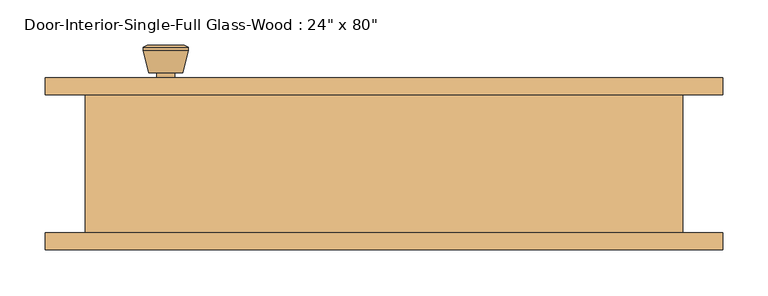
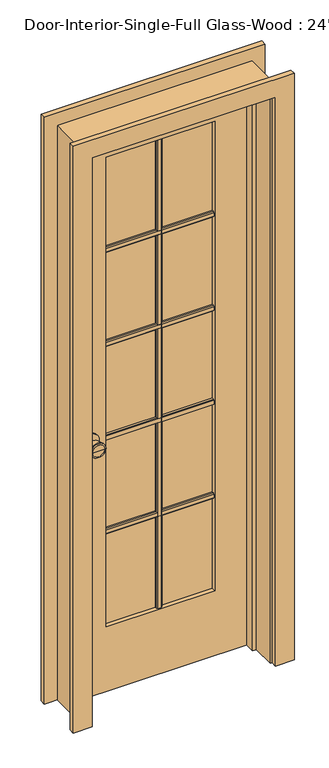
"""IFC4 building model written with IfcOpenShell, lengths in millimetres: door geometry."""

from ifc_helpers import new_model, si_unit, point, frame, frame_2d, origin, place, context, project, spatial, polyline, circle_curve, trimmed, segment, composite_curve, outline, extrude, faceted_brep, source, transform, mapped, element, save
from ifc_brep_helpers import plane_surface, cylinder_surface, revolved_surface, advanced_brep


def door_921d1c85(model_context):
    return source(origin(), model_context, "Body", "SolidModel", [
        extrude(outline(polyline([(59.055, 1586.23), (65.405, 1586.23), (68.58, 1583.055), (68.58, 1570.355), (65.405, 1567.18), (59.055, 1567.18), (59.055, 1586.23)])), frame((-184.15, 0.0, 0.0), z_axis=(1.0, 0.0, 0.0), x_axis=(0.0, 1.0, 0.0)), (0.0, 0.0, 1.0), 368.3),
        extrude(outline(polyline([(59.055, 1249.9975), (65.405, 1249.9975), (68.58, 1246.8225), (68.58, 1234.1225), (65.405, 1230.9475), (59.055, 1230.9475), (59.055, 1249.9975)])), frame((-184.15, 0.0, 0.0), z_axis=(1.0, 0.0, 0.0), x_axis=(0.0, 1.0, 0.0)), (0.0, 0.0, 1.0), 368.3),
        extrude(outline(polyline([(59.055, 913.765), (65.405, 913.765), (68.58, 910.59), (68.58, 897.89), (65.405, 894.715), (59.055, 894.715), (59.055, 913.765)])), frame((-184.15, 0.0, 0.0), z_axis=(1.0, 0.0, 0.0), x_axis=(0.0, 1.0, 0.0)), (0.0, 0.0, 1.0), 368.3),
        extrude(outline(polyline([(-9.525, 59.055), (-9.525, 65.405), (-6.35, 68.58), (6.35, 68.58), (9.525, 65.405), (9.525, 59.055), (-9.525, 59.055)])), frame((0.0, 0.0, 231.775), z_axis=(0.0, 0.0, 1.0), x_axis=(1.0, 0.0, 0.0)), (0.0, 0.0, 1.0), 1681.1625),
        extrude(outline(polyline([(59.055, 577.5325), (65.405, 577.5325), (68.58, 574.3575), (68.58, 561.6575), (65.405, 558.4825), (59.055, 558.4825), (59.055, 577.5325)])), frame((-184.15, 0.0, 0.0), z_axis=(1.0, 0.0, 0.0), x_axis=(0.0, 1.0, 0.0)), (0.0, 0.0, 1.0), 368.3),
        extrude(outline(polyline([(52.07, 1586.23), (52.07, 1567.18), (45.72, 1567.18), (42.545, 1570.355), (42.545, 1583.055), (45.72, 1586.23), (52.07, 1586.23)])), frame((-184.15, 0.0, 0.0), z_axis=(1.0, 0.0, 0.0), x_axis=(0.0, 1.0, 0.0)), (0.0, 0.0, 1.0), 368.3),
        extrude(outline(polyline([(52.07, 1249.9975), (52.07, 1230.9475), (45.72, 1230.9475), (42.545, 1234.1225), (42.545, 1246.8225), (45.72, 1249.9975), (52.07, 1249.9975)])), frame((-184.15, 0.0, 0.0), z_axis=(1.0, 0.0, 0.0), x_axis=(0.0, 1.0, 0.0)), (0.0, 0.0, 1.0), 368.3),
        extrude(outline(polyline([(52.07, 913.765), (52.07, 894.715), (45.72, 894.715), (42.545, 897.89), (42.545, 910.59), (45.72, 913.765), (52.07, 913.765)])), frame((-184.15, 0.0, 0.0), z_axis=(1.0, 0.0, 0.0), x_axis=(0.0, 1.0, 0.0)), (0.0, 0.0, 1.0), 368.3),
        extrude(outline(polyline([(-9.525, 52.07), (9.525, 52.07), (9.525, 45.72), (6.35, 42.545), (-6.35, 42.545), (-9.525, 45.72), (-9.525, 52.07)])), frame((0.0, 0.0, 231.775), z_axis=(0.0, 0.0, 1.0), x_axis=(1.0, 0.0, 0.0)), (0.0, 0.0, 1.0), 1681.1625),
        extrude(outline(polyline([(52.07, 577.5325), (52.07, 558.4825), (45.72, 558.4825), (42.545, 561.6575), (42.545, 574.3575), (45.72, 577.5325), (52.07, 577.5325)])), frame((-184.15, 0.0, 0.0), z_axis=(1.0, 0.0, 0.0), x_axis=(0.0, 1.0, 0.0)), (0.0, 0.0, 1.0), 368.3),
        advanced_brep(
        [(-241.3, 32.1, 914.4), (-231.3, 32.1, 914.4), (-251.3, 32.1, 914.4), (-220.8241324, -16.9, 914.4), (-241.3, -16.9, 914.4), (-261.7758676, -16.9, 914.4), (-216.3, -15.0721319, 914.4), (-266.3, -15.0721319, 914.4), (-216.3, -11.6084537, 914.4), (-266.3, -11.6084537, 914.4), (-222.663764, 13.1, 914.4), (-259.936236, 13.1, 914.4), (-231.3, 13.1, 914.4), (-251.3, 13.1, 914.4)],
        [
            (0, 1),
            (1, 2, circle_curve(frame((-241.3, 32.1, 914.4), z_axis=(0.0, 1.0, 0.0), x_axis=(-1.0, 0.0, 0.0)), 10.0)),
            (2, 0),
            (2, 1, circle_curve(frame((-241.3, 32.1, 914.4), z_axis=(0.0, 1.0, 0.0), x_axis=(-1.0, 0.0, 0.0)), 10.0)),
            (3, 4),
            (4, 5),
            (5, 3, circle_curve(frame((-241.3, -16.9, 914.4), z_axis=(0.0, -1.0, 0.0), x_axis=(-1.0, 0.0, 0.0)), 20.4758676)),
            (3, 5, circle_curve(frame((-241.3, -16.9, 914.4), z_axis=(0.0, -1.0, 0.0), x_axis=(-1.0, 0.0, 0.0)), 20.4758676)),
            (6, 3),
            (5, 7),
            (7, 6, circle_curve(frame((-241.3, -15.0721319, 914.4), z_axis=(0.0, -1.0, 0.0), x_axis=(-1.0, 0.0, 0.0)), 25.0)),
            (6, 7, circle_curve(frame((-241.3, -15.0721319, 914.4), z_axis=(0.0, -1.0, 0.0), x_axis=(-1.0, 0.0, 0.0)), 25.0)),
            (8, 6),
            (7, 9),
            (9, 8, circle_curve(frame((-241.3, -11.6084537, 914.4), z_axis=(0.0, -1.0, 0.0), x_axis=(-1.0, 0.0, 0.0)), 25.0)),
            (8, 9, circle_curve(frame((-241.3, -11.6084537, 914.4), z_axis=(0.0, -1.0, 0.0), x_axis=(-1.0, 0.0, 0.0)), 25.0)),
            (10, 8),
            (9, 11),
            (11, 10, circle_curve(frame((-241.3, 13.1, 914.4), z_axis=(0.0, -1.0, 0.0), x_axis=(-1.0, 0.0, 0.0)), 18.636236)),
            (10, 11, circle_curve(frame((-241.3, 13.1, 914.4), z_axis=(0.0, -1.0, 0.0), x_axis=(-1.0, 0.0, 0.0)), 18.636236)),
            (12, 10),
            (11, 13),
            (13, 12, circle_curve(frame((-241.3, 13.1, 914.4), z_axis=(0.0, -1.0, 0.0), x_axis=(-1.0, 0.0, 0.0)), 10.0)),
            (12, 13, circle_curve(frame((-241.3, 13.1, 914.4), z_axis=(0.0, -1.0, 0.0), x_axis=(-1.0, 0.0, 0.0)), 10.0)),
            (1, 12),
            (13, 2),
        ],
        [
            plane_surface(frame((-241.3, 32.1, 914.4), z_axis=(0.0, 1.0, 0.0), x_axis=(-1.0, 0.0, 0.0))),
            plane_surface(frame((-241.3, -16.9, 914.4), z_axis=(0.0, -1.0, 0.0), x_axis=(-1.0, 0.0, 0.0))),
            revolved_surface(polyline([(-261.7758676, -16.9, 914.4), (-266.3, -15.0721319, 914.4)]), (-241.3, 32.1, 914.4), (0.0, 1.0, 0.0)),
            cylinder_surface(frame((-241.3, 32.1, 914.4), z_axis=(0.0, 1.0, 0.0), x_axis=(-1.0, 0.0, 0.0)), 25.0),
            revolved_surface(polyline([(-266.3, -11.6084537, 914.4), (-259.936236, 13.1, 914.4)]), (-241.3, 32.1, 914.4), (0.0, 1.0, 0.0)),
            plane_surface(frame((-241.3, 13.1, 914.4), z_axis=(0.0, 1.0, 0.0), x_axis=(-1.0, 0.0, 0.0))),
            cylinder_surface(frame((-241.3, 32.1, 914.4), z_axis=(0.0, 1.0, 0.0), x_axis=(-1.0, 0.0, 0.0)), 10.0),
        ],
        [
            (0, [[1, 2, 3]]),
            (0, [[-3, 4, -1]]),
            (1, [[5, 6, 7]]),
            (1, [[-6, -5, 8]]),
            (2, [[9, -7, 10, 11]]),
            (2, [[-10, -8, -9, 12]]),
            (3, [[13, -11, 14, 15]]),
            (3, [[-14, -12, -13, 16]]),
            (4, [[17, -15, 18, 19]]),
            (4, [[-18, -16, -17, 20]]),
            (5, [[21, -19, 22, 23]]),
            (5, [[-22, -20, -21, 24]]),
            (6, [[25, -23, 26, -2]]),
            (6, [[-26, -24, -25, -4]]),
        ],
    ),
        extrude(outline(composite_curve([segment(trimmed(circle_curve(frame_2d((914.4, -241.3)), 30.0), [point((914.4, -271.3))], [point((914.4, -211.3))], False, "CARTESIAN"), True, "CONTINUOUS"), segment(trimmed(circle_curve(frame_2d((914.4, -241.3)), 30.0), [point((914.4, -211.3))], [point((914.4, -271.3))], False, "CARTESIAN"), True, "CONTINUOUS")], self_intersect=False)), frame((0.0, 32.1, 0.0), z_axis=(0.0, 1.0, 0.0), x_axis=(0.0, 0.0, 1.0)), (0.0, 0.0, 1.0), 6.0),
        advanced_brep(
        [(-241.3, 79.025, 914.4), (-251.3, 79.025, 914.4), (-231.3, 79.025, 914.4), (-220.8241324, 128.025, 914.4), (-261.7758676, 128.025, 914.4), (-241.3, 128.025, 914.4), (-216.3, 126.1971319, 914.4), (-266.3, 126.1971319, 914.4), (-216.3, 122.7334537, 914.4), (-266.3, 122.7334537, 914.4), (-222.663764, 98.025, 914.4), (-259.936236, 98.025, 914.4), (-231.3, 98.025, 914.4), (-251.3, 98.025, 914.4)],
        [
            (0, 1),
            (1, 2, circle_curve(frame((-241.3, 79.025, 914.4), z_axis=(0.0, -1.0, 0.0), x_axis=(-1.0, 0.0, 0.0)), 10.0)),
            (2, 0),
            (2, 1, circle_curve(frame((-241.3, 79.025, 914.4), z_axis=(0.0, -1.0, 0.0), x_axis=(-1.0, 0.0, 0.0)), 10.0)),
            (3, 4, circle_curve(frame((-241.3, 128.025, 914.4), z_axis=(0.0, 1.0, 0.0), x_axis=(-1.0, 0.0, 0.0)), 20.4758676)),
            (4, 5),
            (5, 3),
            (4, 3, circle_curve(frame((-241.3, 128.025, 914.4), z_axis=(0.0, 1.0, 0.0), x_axis=(-1.0, 0.0, 0.0)), 20.4758676)),
            (6, 7, circle_curve(frame((-241.3, 126.1971319, 914.4), z_axis=(0.0, 1.0, 0.0), x_axis=(-1.0, 0.0, 0.0)), 25.0)),
            (7, 4),
            (3, 6),
            (7, 6, circle_curve(frame((-241.3, 126.1971319, 914.4), z_axis=(0.0, 1.0, 0.0), x_axis=(-1.0, 0.0, 0.0)), 25.0)),
            (8, 9, circle_curve(frame((-241.3, 122.7334537, 914.4), z_axis=(0.0, 1.0, 0.0), x_axis=(-1.0, 0.0, 0.0)), 25.0)),
            (9, 7),
            (6, 8),
            (9, 8, circle_curve(frame((-241.3, 122.7334537, 914.4), z_axis=(0.0, 1.0, 0.0), x_axis=(-1.0, 0.0, 0.0)), 25.0)),
            (10, 11, circle_curve(frame((-241.3, 98.025, 914.4), z_axis=(0.0, 1.0, 0.0), x_axis=(-1.0, 0.0, 0.0)), 18.636236)),
            (11, 9),
            (8, 10),
            (11, 10, circle_curve(frame((-241.3, 98.025, 914.4), z_axis=(0.0, 1.0, 0.0), x_axis=(-1.0, 0.0, 0.0)), 18.636236)),
            (12, 13, circle_curve(frame((-241.3, 98.025, 914.4), z_axis=(0.0, 1.0, 0.0), x_axis=(-1.0, 0.0, 0.0)), 10.0)),
            (13, 11),
            (10, 12),
            (13, 12, circle_curve(frame((-241.3, 98.025, 914.4), z_axis=(0.0, 1.0, 0.0), x_axis=(-1.0, 0.0, 0.0)), 10.0)),
            (1, 13),
            (12, 2),
        ],
        [
            plane_surface(frame((-241.3, 79.025, 914.4), z_axis=(0.0, -1.0, 0.0), x_axis=(-1.0, 0.0, 0.0))),
            plane_surface(frame((-241.3, 128.025, 914.4), z_axis=(0.0, 1.0, 0.0), x_axis=(-1.0, 0.0, 0.0))),
            revolved_surface(polyline([(-261.7758676, 128.025, 914.4), (-266.3, 126.1971319, 914.4)]), (-241.3, 79.025, 914.4), (0.0, -1.0, 0.0)),
            cylinder_surface(frame((-241.3, 79.025, 914.4), z_axis=(0.0, -1.0, 0.0), x_axis=(-1.0, 0.0, 0.0)), 25.0),
            revolved_surface(polyline([(-266.3, 122.7334537, 914.4), (-259.936236, 98.025, 914.4)]), (-241.3, 79.025, 914.4), (0.0, -1.0, 0.0)),
            plane_surface(frame((-241.3, 98.025, 914.4), z_axis=(0.0, -1.0, 0.0), x_axis=(-1.0, 0.0, 0.0))),
            cylinder_surface(frame((-241.3, 79.025, 914.4), z_axis=(0.0, -1.0, 0.0), x_axis=(-1.0, 0.0, 0.0)), 10.0),
        ],
        [
            (0, [[1, 2, 3]]),
            (0, [[-3, 4, -1]]),
            (1, [[5, 6, 7]]),
            (1, [[8, -7, -6]]),
            (2, [[9, 10, -5, 11]]),
            (2, [[12, -11, -8, -10]]),
            (3, [[13, 14, -9, 15]]),
            (3, [[16, -15, -12, -14]]),
            (4, [[17, 18, -13, 19]]),
            (4, [[20, -19, -16, -18]]),
            (5, [[21, 22, -17, 23]]),
            (5, [[24, -23, -20, -22]]),
            (6, [[-2, 25, -21, 26]]),
            (6, [[-4, -26, -24, -25]]),
        ],
    ),
        extrude(outline(composite_curve([segment(trimmed(circle_curve(frame_2d((914.4, -241.3)), 30.0), [point((914.4, -271.3))], [point((914.4, -211.3))], False, "CARTESIAN"), True, "CONTINUOUS"), segment(trimmed(circle_curve(frame_2d((914.4, -241.3)), 30.0), [point((914.4, -211.3))], [point((914.4, -271.3))], False, "CARTESIAN"), True, "CONTINUOUS")], self_intersect=False)), frame((0.0, 73.025, 0.0), z_axis=(0.0, 1.0, 0.0), x_axis=(0.0, 0.0, 1.0)), (0.0, 0.0, 1.0), 6.0),
        extrude(outline(polyline([(2032.0, -304.8), (0.0, -304.8), (0.0, 304.8), (2032.0, 304.8), (2032.0, -304.8)]), holes=[polyline([(1912.9375, -184.15), (1912.9375, 184.15), (231.775, 184.15), (231.775, -184.15), (1912.9375, -184.15)])]), frame((0.0, 38.1, 0.0), z_axis=(0.0, 1.0, 0.0), x_axis=(0.0, 0.0, 1.0)), (0.0, 0.0, 1.0), 34.925),
        faceted_brep([(330.2, 73.025, 0.0), (330.2, -79.375, 0.0), (304.8, -79.375, 0.0), (304.8, 3.175, 0.0), (292.1, 3.175, 0.0), (292.1, 38.1, 0.0), (304.8, 38.1, 0.0), (304.8, 73.025, 0.0), (330.2, 73.025, 2057.4), (330.2, -79.375, 2057.4), (-330.2, -79.375, 2057.4), (-330.2, -79.375, 0.0), (-304.8, -79.375, 0.0), (-304.8, -79.375, 2032.0), (304.8, -79.375, 2032.0), (304.8, 3.175, 2032.0), (-304.8, 3.175, 2032.0), (-304.8, 3.175, 0.0), (-292.1, 3.175, 0.0), (-292.1, 3.175, 2019.3), (292.1, 3.175, 2019.3), (292.1, 38.1, 2019.3), (-292.1, 38.1, 2019.3), (-292.1, 38.1, 0.0), (-304.8, 38.1, 0.0), (-304.8, 38.1, 2032.0), (304.8, 38.1, 2032.0), (304.8, 73.025, 2032.0), (-304.8, 73.025, 2032.0), (-304.8, 73.025, 0.0), (-330.2, 73.025, 0.0), (-330.2, 73.025, 2057.4)], [[[0, 1, 2, 3, 4, 5, 6, 7]], [[1, 0, 8, 9]], [[2, 1, 9, 10, 11, 12, 13, 14]], [[3, 2, 14, 15]], [[4, 3, 15, 16, 17, 18, 19, 20]], [[5, 4, 20, 21]], [[6, 5, 21, 22, 23, 24, 25, 26]], [[7, 6, 26, 27]], [[0, 7, 27, 28, 29, 30, 31, 8]], [[9, 8, 31, 10]], [[15, 14, 13, 16]], [[21, 20, 19, 22]], [[27, 26, 25, 28]], [[30, 29, 24, 23, 18, 17, 12, 11]], [[10, 31, 30, 11]], [[16, 13, 12, 17]], [[22, 19, 18, 23]], [[28, 25, 24, 29]]]),
        extrude(outline(polyline([(184.15, 52.07), (-184.15, 52.07), (-184.15, 59.055), (184.15, 59.055), (184.15, 52.07)])), frame((0.0, 0.0, 231.775), z_axis=(0.0, 0.0, 1.0), x_axis=(1.0, 0.0, 0.0)), (0.0, 0.0, 1.0), 1681.1625),
        extrude(outline(polyline([(0.0, 311.15), (0.0, 374.65), (2101.85, 374.65), (2101.85, -374.65), (0.0, -374.65), (0.0, -311.15), (2038.35, -311.15), (2038.35, 311.15), (0.0, 311.15)])), frame((0.0, -98.425, 0.0), z_axis=(0.0, 1.0, 0.0), x_axis=(0.0, 0.0, 1.0)), (0.0, 0.0, 1.0), 19.05),
        extrude(outline(polyline([(0.0, 311.15), (0.0, 374.65), (2101.85, 374.65), (2101.85, -374.65), (0.0, -374.65), (0.0, -311.15), (2038.35, -311.15), (2038.35, 311.15), (0.0, 311.15)])), frame((0.0, 73.025, 0.0), z_axis=(0.0, 1.0, 0.0), x_axis=(0.0, 0.0, 1.0)), (0.0, 0.0, 1.0), 19.05),
    ])


if __name__ == "__main__":
    model = new_model("IFC4")
    model_context = context("Model", 3, world=origin())
    ifc_project = project(units=[si_unit("LENGTHUNIT", "METRE", prefix="MILLI")], contexts=[model_context])
    site = spatial("IfcSite", under=ifc_project)
    building = spatial("IfcBuilding", under=site)
    placement = place(None, origin())
    door_shape = door_921d1c85(model_context)
    element("IfcDoor", 1, ObjectType="Door-Interior-Single-Full Glass-Wood : 24\" x 80\"", at=placement, inside=building, context=model_context, shape_type="MappedRepresentation", body=[
        mapped(door_shape, transform((0.0, 0.0, 0.0), x_axis=(1.0, 0.0, 0.0), y_axis=(0.0, 1.0, 0.0), z_axis=(0.0, 0.0, 1.0))),
    ])
    save(model, "model.ifc")

# Revit data of these elements
# Type "Door-Interior-Single-Full Glass-Wood : 24\" x 80\""
#   Type Mark = "10"
#   Assembly Code = "C1020300"
#   Analytic Construction = "Wood frame with single clear glass"
#   Top Rail = 0' - 4 11/16"
#   Thickness = 0' - 1 3/8"
#   Thermal Resistance (R) = 1.0102 (h·ft²·°F)/BTU
#   Swing Angle [instance default] = 90.00°
#   Stiles = 0' - 4 3/4"
#   Rough Width = 2' - 2"
#   Rough Height = 6' - 9"
#   Height = 6' - 8"
#   Width = 2' - 0"
#   Heat Transfer Coefficient (U) = 0.9900 BTU/(h·ft²·°F)
#   Bottom Rail = 0' - 9 1/8"
#   Show Grill [instance default] = yes
#   Trim Material = Cherry
#   Panel Material = Cherry
#   Frame Material = Cherry
#   Door Handle Material = Aluminum
#   Visual Light Transmittance = 0
#   Solar Heat Gain Coefficient = 0
#   Wall Closure = (empty or 0)
#   Function = (empty or 0)
# Element 1 (IfcDoor, "Door-Interior-Single-Full Glass-Wood : 24\" x 80\"")
#   Materials on its faces: "Cherry", "Aluminum", "Glass"
# Materials
#   "Cherry": class "Wood", colour RGB 226 177 128, transparency 0, Description = "Prunus Serotina", Cost = 0
#   "Aluminum": class "Metal", colour RGB 247 247 247, transparency 0, Description = "Aluminum 6061", Cost = 0
#   "Glass": class "Glass", colour RGB 0 128 192, transparency 0.75, Description = "Soda Lime Glass", Cost = 0
